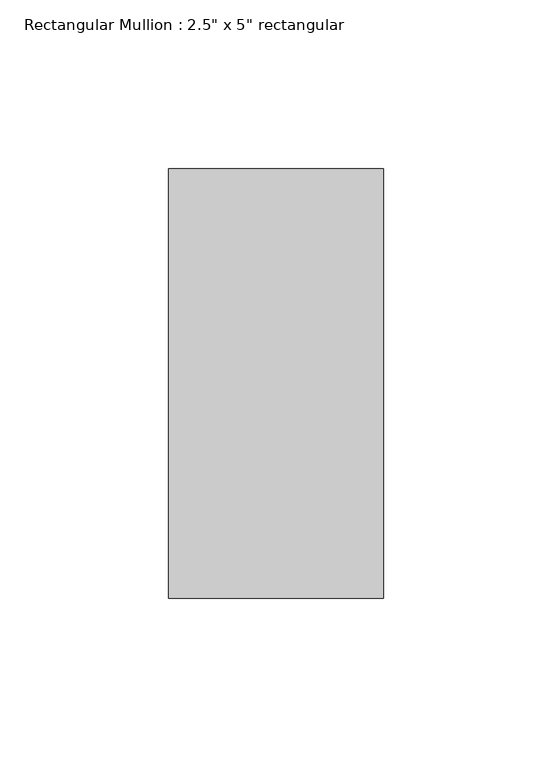
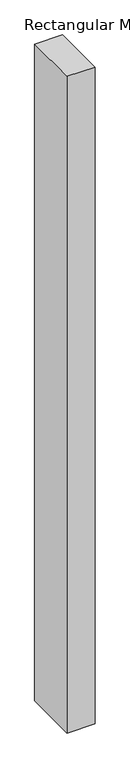
"""IFC4 building model written with IfcOpenShell, lengths in millimetres: member geometry."""

from ifc_helpers import new_model, si_unit, frame, origin, place, context, project, spatial, polyline, outline, extrude, source, transform, mapped, element, save


def member_2820fca8(model_context):
    return source(origin(), model_context, "Body", "SweptSolid", [
        extrude(outline(polyline([(31.75, 63.5), (31.75, -63.5), (-31.75, -63.5), (-31.75, 63.5), (31.75, 63.5)])), frame((0.0, 0.0, -1570.4687519), z_axis=(0.0, 0.0, 1.0), x_axis=(1.0, 0.0, 0.0)), (0.0, 0.0, 1.0), 1570.4687519),
    ])


if __name__ == "__main__":
    model = new_model("IFC4")
    model_context = context("Model", 3, world=origin())
    ifc_project = project(units=[si_unit("LENGTHUNIT", "METRE", prefix="MILLI")], contexts=[model_context])
    site = spatial("IfcSite", under=ifc_project)
    building = spatial("IfcBuilding", under=site)
    placement = place(None, origin())
    member_shape = member_2820fca8(model_context)
    element("IfcMember", 1, ObjectType="Rectangular Mullion : 2.5\" x 5\" rectangular", at=placement, inside=building, context=model_context, shape_type="MappedRepresentation", body=[
        mapped(member_shape, transform((0.0, 0.0, 0.0), x_axis=(1.0, 0.0, 0.0), y_axis=(0.0, 1.0, 0.0), z_axis=(0.0, 0.0, 1.0))),
    ])
    save(model, "model.ifc")

# Revit data of these elements
# Type "Rectangular Mullion : 2.5\" x 5\" rectangular"
#   built-in parameter 1007304 = 0.416667 (stored number, unit not read)
#   built-in parameter 1007301 = 0.104167 (stored number, unit not read)
#   built-in parameter 1007300 = 0.104167 (stored number, unit not read)
# Element 1 (IfcMember, "Rectangular Mullion : 2.5\" x 5\" rectangular")
#   Materials on its faces: "Aluminum"
# Materials
#   "Aluminum": class "Metal", colour RGB 247 247 247, transparency 0, Description = "Aluminum 6061", Cost = 0
